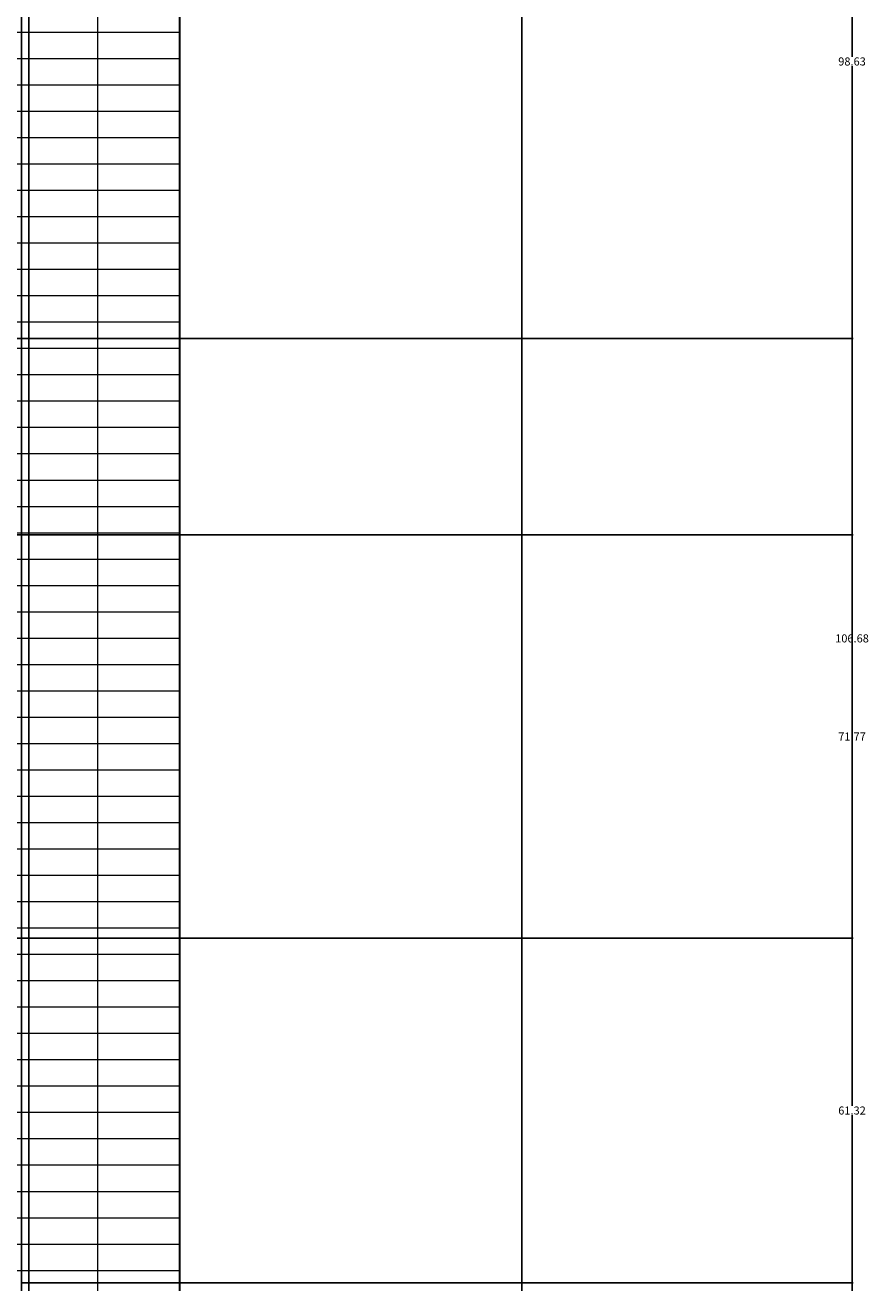
# Model space of a CAD drawing. Units: inches. Extents: x 241 to 943, y 109 to 1396.
# Tile 28 of 34: x 793 to 943, y 842 to 1065. Entities that reach past the tile are written whole.
import ezdxf

# ---------------------------------------------------------------- set-up
doc = ezdxf.new("R2010")
doc.units = ezdxf.units.IN
doc.header["$MEASUREMENT"] = 0
for name, color, linetype, lineweight in [('A-ANNO-DIMS', 2, 'Continuous', 18), ('A-ELEV', 7, 'Continuous', 25), ('A-WALL-PATT', 8, 'Continuous', 13)]:
    doc.layers.add(name, color=color, linetype=linetype, lineweight=lineweight)
doc.styles.get("Standard").update_dxf_attribs({"font": 'arial.ttf'})
doc.dimstyles.get("Standard").update_dxf_attribs({"dimtxt": 1.4375, "dimasz": 0.18, "dimexe": 0.18, "dimexo": 0.0625, "dimgap": 0.09, "dimtad": 0, "dimtih": 1, "dimtoh": 1, "dimdec": 4, "dimzin": 0, "dimdsep": 46, "dimlunit": 4, "dimtxsty": 'Standard', "dimcen": 0.09, "dimadec": 0, "dimazin": 0, "dimtfac": 1, "dimtdec": 4, "dimtofl": 0, "dimtmove": 0, "dimatfit": 3, "dimfxl": 1, "dimtolj": 1, "dimtzin": 0, "dimarcsym": 0})

# ---------------------------------------------------------------- blocks, each defined once
blk = doc.blocks.new('*D6')
at = {"layer": 'A-ANNO-DIMS', "color": 0, "lineweight": -2, "transparency": 16777216}
for p, q in [((820.84, 232.89), (820.84, 1395.05)), ((821.02, 1394.87), (848.73, 1394.87)), ((881.49, 1394.87), (853.77, 1394.87)), ((881.67, 232.89), (881.67, 1395.05))]:
    blk.add_line(p, q, dxfattribs=at)
at = {"layer": 'A-ANNO-DIMS', "color": 0, "transparency": 16777216}
for points in [[(821.02, 1394.9), (821.02, 1394.84), (820.84, 1394.87)], [(881.49, 1394.9), (881.49, 1394.84), (881.67, 1394.87)]]:
    blk.add_solid(points, dxfattribs=at)
at = {"layer": 'Defpoints', "color": 0, "transparency": 16777216}
for p in [(881.67, 1394.87), (820.84, 232.83), (881.67, 232.83)]:
    blk.add_point(p, dxfattribs=at)
at = {"layer": 'A-ANNO-DIMS', "color": 0, "transparency": 16777216, "insert": (851.25, 1394.87), "char_height": 1.438, "attachment_point": 5}
blk.add_mtext('\\A1;60.83', dxfattribs=at)
blk = doc.blocks.new('*D14')
at = {"layer": 'A-ANNO-DIMS', "color": 0, "lineweight": -2, "transparency": 16777216}
for p, q in [((667.39, 290.06), (667.39, 1395.05)), ((667.57, 1394.87), (727.7, 1394.87)), ((793.85, 1394.87), (733.72, 1394.87)), ((794.03, 290.06), (794.03, 1395.05))]:
    blk.add_line(p, q, dxfattribs=at)
at = {"layer": 'A-ANNO-DIMS', "color": 0, "transparency": 16777216}
for points in [[(667.57, 1394.9), (667.57, 1394.84), (667.39, 1394.87)], [(793.85, 1394.9), (793.85, 1394.84), (794.03, 1394.87)]]:
    blk.add_solid(points, dxfattribs=at)
at = {"layer": 'Defpoints', "color": 0, "transparency": 16777216}
for p in [(794.03, 1394.87), (667.39, 290), (794.03, 290)]:
    blk.add_point(p, dxfattribs=at)
at = {"layer": 'A-ANNO-DIMS', "color": 0, "transparency": 16777216, "insert": (730.71, 1394.87), "char_height": 1.438, "attachment_point": 5}
blk.add_mtext('\\A1;126.63', dxfattribs=at)
blk = doc.blocks.new('*D15')
at = {"layer": 'A-ANNO-DIMS', "color": 0, "lineweight": -2, "transparency": 16777216}
for p, q in [((794.03, 290.06), (794.03, 1395.05)), ((794.21, 1394.87), (805.04, 1394.87)), ((820.66, 1394.87), (809.82, 1394.87)), ((820.84, 232.89), (820.84, 1395.05))]:
    blk.add_line(p, q, dxfattribs=at)
at = {"layer": 'A-ANNO-DIMS', "color": 0, "transparency": 16777216}
for points in [[(794.21, 1394.9), (794.21, 1394.84), (794.03, 1394.87)], [(820.66, 1394.9), (820.66, 1394.84), (820.84, 1394.87)]]:
    blk.add_solid(points, dxfattribs=at)
at = {"layer": 'Defpoints', "color": 0, "transparency": 16777216}
for p in [(820.84, 1394.87), (794.03, 290), (820.84, 232.83)]:
    blk.add_point(p, dxfattribs=at)
at = {"layer": 'A-ANNO-DIMS', "color": 0, "transparency": 16777216, "insert": (807.43, 1394.87), "char_height": 1.438, "attachment_point": 5}
blk.add_mtext('\\A1;26.81', dxfattribs=at)
blk = doc.blocks.new('*D47')
at = {"layer": 'A-ANNO-DIMS', "color": 0, "lineweight": -2, "transparency": 16777216}
for p, q in [((792.75, 841.54), (940.6, 841.54)), ((940.42, 841.36), (940.42, 789.02)), ((940.42, 735.03), (940.42, 787.37)), ((792.75, 734.85), (940.6, 734.85))]:
    blk.add_line(p, q, dxfattribs=at)
at = {"layer": 'A-ANNO-DIMS', "color": 0, "transparency": 16777216}
for points in [[(940.39, 841.36), (940.45, 841.36), (940.42, 841.54)], [(940.39, 735.03), (940.45, 735.03), (940.42, 734.85)]]:
    blk.add_solid(points, dxfattribs=at)
at = {"layer": 'Defpoints', "color": 0, "transparency": 16777216}
for p in [(792.69, 841.54), (940.42, 841.54), (792.69, 734.85)]:
    blk.add_point(p, dxfattribs=at)
at = {"layer": 'A-ANNO-DIMS', "color": 0, "transparency": 16777216, "insert": (940.42, 788.2), "char_height": 1.438, "attachment_point": 5}
blk.add_mtext('\\A1;106.68', dxfattribs=at)
blk = doc.blocks.new('*D48')
at = {"layer": 'A-ANNO-DIMS', "color": 0, "lineweight": -2, "transparency": 16777216}
for p, q in [((751.57, 1009.54), (940.6, 1009.54)), ((940.42, 1009.36), (940.42, 957.02)), ((940.42, 903.03), (940.42, 955.37)), ((751.57, 902.85), (940.6, 902.85))]:
    blk.add_line(p, q, dxfattribs=at)
at = {"layer": 'A-ANNO-DIMS', "color": 0, "transparency": 16777216}
for points in [[(940.39, 1009.36), (940.45, 1009.36), (940.42, 1009.54)], [(940.39, 903.03), (940.45, 903.03), (940.42, 902.85)]]:
    blk.add_solid(points, dxfattribs=at)
at = {"layer": 'Defpoints', "color": 0, "transparency": 16777216}
for p in [(751.51, 1009.54), (940.42, 1009.54), (751.51, 902.85)]:
    blk.add_point(p, dxfattribs=at)
at = {"layer": 'A-ANNO-DIMS', "color": 0, "transparency": 16777216, "insert": (940.42, 956.2), "char_height": 1.438, "attachment_point": 5}
blk.add_mtext('\\A1;106.68', dxfattribs=at)
blk = doc.blocks.new('*D64')
at = {"layer": 'A-ANNO-DIMS', "color": 0, "lineweight": -2, "transparency": 16777216}
for p, q in [((792.69, 568.89), (792.69, 1395.05)), ((792.87, 1394.87), (803.68, 1394.87)), ((820.66, 1394.87), (809.85, 1394.87)), ((820.84, 568.89), (820.84, 1395.05))]:
    blk.add_line(p, q, dxfattribs=at)
at = {"layer": 'A-ANNO-DIMS', "color": 0, "transparency": 16777216}
for points in [[(792.87, 1394.9), (792.87, 1394.84), (792.69, 1394.87)], [(820.66, 1394.9), (820.66, 1394.84), (820.84, 1394.87)]]:
    blk.add_solid(points, dxfattribs=at)
at = {"layer": 'Defpoints', "color": 0, "transparency": 16777216}
for p in [(820.84, 1394.87), (792.69, 568.83), (820.84, 568.83)]:
    blk.add_point(p, dxfattribs=at)
at = {"layer": 'A-ANNO-DIMS', "color": 0, "transparency": 16777216, "insert": (806.76, 1394.87), "char_height": 1.438, "attachment_point": 5}
blk.add_mtext('\\A1;28.146', dxfattribs=at)
blk = doc.blocks.new('*D71')
at = {"layer": 'A-ANNO-DIMS', "color": 0, "lineweight": -2, "transparency": 16777216}
for p, q in [((751.51, 902.92), (751.51, 1395.05)), ((751.69, 1394.87), (783.65, 1394.87)), ((820.66, 1394.87), (788.69, 1394.87)), ((820.84, 902.92), (820.84, 1395.05))]:
    blk.add_line(p, q, dxfattribs=at)
at = {"layer": 'A-ANNO-DIMS', "color": 0, "transparency": 16777216}
for points in [[(751.69, 1394.9), (751.69, 1394.84), (751.51, 1394.87)], [(820.66, 1394.9), (820.66, 1394.84), (820.84, 1394.87)]]:
    blk.add_solid(points, dxfattribs=at)
at = {"layer": 'Defpoints', "color": 0, "transparency": 16777216}
for p in [(820.84, 1394.87), (751.51, 902.85), (820.84, 902.85)]:
    blk.add_point(p, dxfattribs=at)
at = {"layer": 'A-ANNO-DIMS', "color": 0, "transparency": 16777216, "insert": (786.17, 1394.87), "char_height": 1.438, "attachment_point": 5}
blk.add_mtext('\\A1;69.33', dxfattribs=at)
blk = doc.blocks.new('*D84')
at = {"layer": 'A-ANNO-DIMS', "color": 0, "lineweight": -2, "transparency": 16777216}
for p, q in [((749.63, 702.85), (749.63, 1395.05)), ((749.81, 1394.87), (782.73, 1394.87)), ((820.66, 1394.87), (787.74, 1394.87)), ((820.84, 736.89), (820.84, 1395.05))]:
    blk.add_line(p, q, dxfattribs=at)
at = {"layer": 'A-ANNO-DIMS', "color": 0, "transparency": 16777216}
for points in [[(749.81, 1394.9), (749.81, 1394.84), (749.63, 1394.87)], [(820.66, 1394.9), (820.66, 1394.84), (820.84, 1394.87)]]:
    blk.add_solid(points, dxfattribs=at)
at = {"layer": 'Defpoints', "color": 0, "transparency": 16777216}
for p in [(820.84, 1394.87), (820.84, 736.83), (749.63, 702.79)]:
    blk.add_point(p, dxfattribs=at)
at = {"layer": 'A-ANNO-DIMS', "color": 0, "transparency": 16777216, "insert": (785.24, 1394.87), "char_height": 1.438, "attachment_point": 5}
blk.add_mtext('\\A1;71.20', dxfattribs=at)
blk = doc.blocks.new('*D87')
at = {"layer": 'A-ANNO-DIMS', "color": 0, "lineweight": -2, "transparency": 16777216}
for p, q in [((751.57, 902.85), (940.6, 902.85)), ((940.42, 902.67), (940.42, 873.02)), ((940.42, 841.72), (940.42, 871.37)), ((792.75, 841.54), (940.6, 841.54))]:
    blk.add_line(p, q, dxfattribs=at)
at = {"layer": 'A-ANNO-DIMS', "color": 0, "transparency": 16777216}
for points in [[(940.39, 902.67), (940.45, 902.67), (940.42, 902.85)], [(940.39, 841.72), (940.45, 841.72), (940.42, 841.54)]]:
    blk.add_solid(points, dxfattribs=at)
at = {"layer": 'Defpoints', "color": 0, "transparency": 16777216}
for p in [(751.51, 902.85), (940.42, 902.85), (792.69, 841.54)]:
    blk.add_point(p, dxfattribs=at)
at = {"layer": 'A-ANNO-DIMS', "color": 0, "transparency": 16777216, "insert": (940.42, 872.2), "char_height": 1.438, "attachment_point": 5}
blk.add_mtext('\\A1;61.32', dxfattribs=at)
blk = doc.blocks.new('*D88')
at = {"layer": 'A-ANNO-DIMS', "color": 0, "lineweight": -2, "transparency": 16777216}
for p, q in [((724.88, 1108.17), (940.6, 1108.17)), ((940.42, 1107.99), (940.42, 1059.68)), ((940.42, 1009.72), (940.42, 1058.03)), ((751.57, 1009.54), (940.6, 1009.54))]:
    blk.add_line(p, q, dxfattribs=at)
at = {"layer": 'A-ANNO-DIMS', "color": 0, "transparency": 16777216}
for points in [[(940.39, 1107.99), (940.45, 1107.99), (940.42, 1108.17)], [(940.39, 1009.72), (940.45, 1009.72), (940.42, 1009.54)]]:
    blk.add_solid(points, dxfattribs=at)
at = {"layer": 'Defpoints', "color": 0, "transparency": 16777216}
for p in [(724.82, 1108.17), (940.42, 1108.17), (751.51, 1009.54)]:
    blk.add_point(p, dxfattribs=at)
at = {"layer": 'A-ANNO-DIMS', "color": 0, "transparency": 16777216, "insert": (940.42, 1058.85), "char_height": 1.438, "attachment_point": 5}
blk.add_mtext('\\A1;98.63', dxfattribs=at)
blk = doc.blocks.new('*D118')
at = {"layer": 'A-ANNO-DIMS', "color": 0, "lineweight": -2, "transparency": 16777216}
for p, q in [((712.65, 974.63), (940.6, 974.63)), ((940.42, 974.45), (940.42, 939.55)), ((940.42, 903.03), (940.42, 937.93)), ((712.65, 902.85), (940.6, 902.85))]:
    blk.add_line(p, q, dxfattribs=at)
at = {"layer": 'A-ANNO-DIMS', "color": 0, "transparency": 16777216}
for points in [[(940.39, 974.45), (940.45, 974.45), (940.42, 974.63)], [(940.39, 903.03), (940.45, 903.03), (940.42, 902.85)]]:
    blk.add_solid(points, dxfattribs=at)
at = {"layer": 'Defpoints', "color": 0, "transparency": 16777216}
for p in [(712.58, 974.63), (940.42, 974.63), (712.58, 902.85)]:
    blk.add_point(p, dxfattribs=at)
at = {"layer": 'A-ANNO-DIMS', "color": 0, "transparency": 16777216, "insert": (940.42, 938.74), "char_height": 1.438, "attachment_point": 5}
blk.add_mtext('\\A1;71.77', dxfattribs=at)

msp = doc.modelspace()

# ---------------------------------------------------------------- hatches: boundary and pattern name
at = {"layer": 'A-WALL-PATT'}
h = msp.add_hatch(dxfattribs=at)
h.set_pattern_fill('GRATE', color=256, scale=150)
h.paths.add_polyline_path([(820.8374, 1070.8538), (749.6328, 1070.8538), (553.5166, 1070.8538), (508.3064, 1070.8538), (508.3064, 1009.5382), (553.5166, 1009.5382), (564.8076, 1009.5382), (603.8694, 1009.5382), (751.5078, 1009.5382), (751.5078, 902.8538), (603.8694, 902.8538), (603.8694, 1009.5382), (564.8076, 1009.5382), (564.8076, 941.4916), (568.1348, 941.4916), (568.1348, 902.8538), (581.3632, 902.8538), (581.3632, 841.5382), (564.8076, 841.5382), (564.8076, 782.5808), (605.9087, 782.5808, -1), (605.9087, 780.5808), (564.8076, 780.5808), (564.8076, 773.4916), (597.514, 773.4916), (607.8162, 773.4916), (607.8162, 734.8538), (617.7594, 734.8538), (617.7594, 841.5382), (792.691, 841.5382), (792.691, 734.8538), (617.7594, 734.8538), (617.7594, 702.7912), (749.6328, 702.7912), (749.6328, 626.4013), (617.7594, 626.4013), (617.7594, 568.8295), (820.8374, 568.8295), (820.8374, 736.8295), (820.8374, 902.8538)])

# ---------------------------------------------------------------- linework, layer by layer
at = {"layer": 'A-ELEV'}
for p, q in [((820.8374, 902.8538), (820.8374, 1070.8538)), ((820.8374, 736.8295), (820.8374, 902.8538))]:
    msp.add_line(p, q, dxfattribs=at)

# ---------------------------------------------------------------- dimensions: what is measured, and where the dimension line sits
at = {"layer": 'A-ANNO-DIMS'}
for base, p1, p2, override, picture, middle in [((794.0275, 1394.8654), (667.3935, 289.9984), (794.0275, 289.9984), {"dimdec": 2, "dimlfac": 1, "dimrnd": 0, "dimzin": 0, "dimdsep": 46, "dimlunit": 2}, '*D14', (730.7105, 1394.8654)), ((820.8374, 1394.8654), (749.6328, 702.7912), (820.8374, 736.8295), {"dimdec": 2, "dimlfac": 1, "dimrnd": 0, "dimzin": 0, "dimdsep": 46, "dimlunit": 2}, '*D84', (785.2351, 1394.8654)), ((820.8374, 1394.8654), (751.5078, 902.8538), (820.8374, 902.8538), {"dimdec": 2, "dimlfac": 1, "dimrnd": 0, "dimzin": 0, "dimdsep": 46, "dimlunit": 2}, '*D71', (786.1726, 1394.8654)), ((820.8374, 1394.8654), (792.691, 568.8295), (820.8374, 568.8295), {"dimdec": 3, "dimlfac": 1, "dimrnd": 0, "dimzin": 0, "dimdsep": 46, "dimlunit": 2}, '*D64', (806.7642, 1394.8654)), ((820.8374, 1394.8654), (794.0275, 289.9984), (820.8374, 232.8295), {"dimdec": 2, "dimlfac": 1, "dimrnd": 0, "dimzin": 0, "dimdsep": 46, "dimlunit": 2}, '*D15', (807.4324, 1394.8654)), ((881.667, 1394.8654), (820.8374, 232.8295), (881.667, 232.8295), {"dimdec": 2, "dimlfac": 1, "dimrnd": 0, "dimzin": 0, "dimdsep": 46, "dimlunit": 2}, '*D6', (851.2522, 1394.8654))]:
    dim = msp.add_linear_dim(base=base, p1=p1, p2=p2, dimstyle='Standard', override=override, dxfattribs=at)
    dim.commit()
    dim.dimension.update_dxf_attribs({"geometry": picture, "text_midpoint": middle})
for base, p1, p2, picture, middle in [((940.417, 1108.1686), (751.5078, 1009.5382), (724.819, 1108.1686), '*D88', (940.417, 1058.8534)), ((940.417, 1009.5382), (751.5078, 902.8538), (751.5078, 1009.5382), '*D48', (940.417, 956.196)), ((940.417, 974.6275), (712.5839, 902.8538), (712.5839, 974.6275), '*D118', (940.417, 938.7406)), ((940.417, 902.8538), (792.691, 841.5382), (751.5078, 902.8538), '*D87', (940.417, 872.196)), ((940.417, 841.5382), (792.691, 734.8538), (792.691, 841.5382), '*D47', (940.417, 788.196))]:
    dim = msp.add_linear_dim(base=base, p1=p1, p2=p2, angle=90, dimstyle='Standard', override={"dimdec": 2, "dimlfac": 1, "dimrnd": 0, "dimzin": 0, "dimdsep": 46, "dimlunit": 2}, dxfattribs=at)
    dim.commit()
    dim.dimension.update_dxf_attribs({"geometry": picture, "text_midpoint": middle})

doc.saveas('drawing.dxf')
